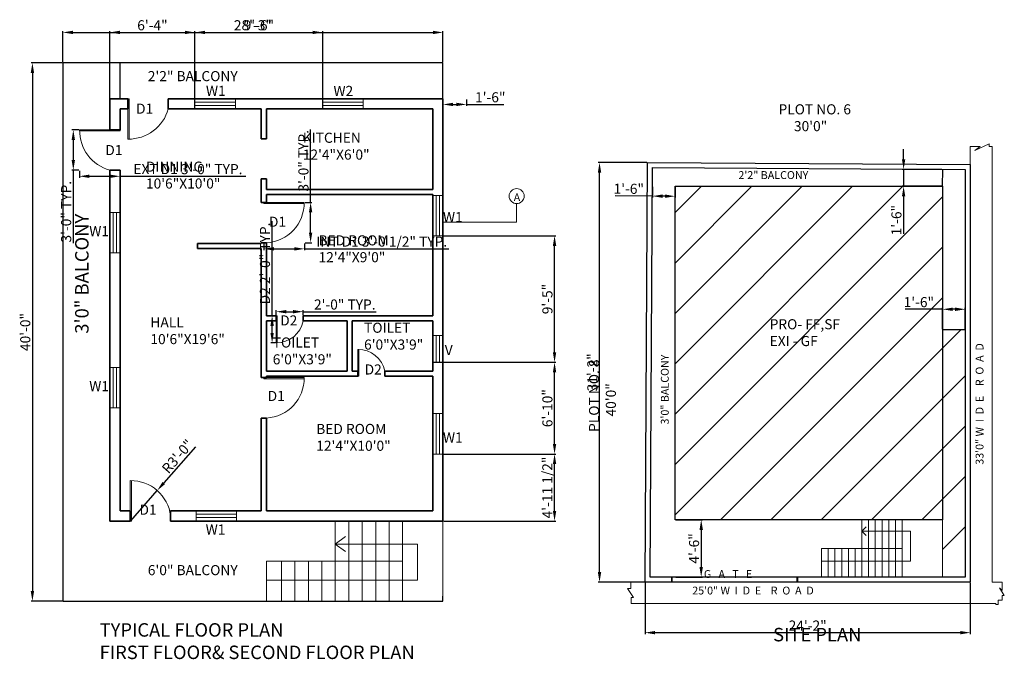
# Model space of a CAD drawing. Units: inches. Extents: x 2044 to 3644, y 808 to 1988.
# Tile 3 of 4: x 2766 to 3644, y 841 to 1412. Entities that reach past the tile are written whole.
import ezdxf

# ---------------------------------------------------------------- set-up
doc = ezdxf.new("R2010")
doc.units = ezdxf.units.IN
for name, color, linetype, lineweight in [('A-ANNO-DIMS', 2, 'Continuous', 18), ('A-ANNO-SYMB', 2, 'Continuous', 18), ('A-ANNO-TEXT', 7, 'Continuous', 18), ('A-ANNO-TITL', 7, 'Continuous', 25), ('A-AREA-IDEN', 7, 'Continuous', 18), ('A-DOOR', 4, 'Continuous', 18), ('A-FLOR-BALC', 7, 'Continuous', 25), ('A-FLOR-STRS', 3, 'Continuous', 18), ('A-GLAZ', 4, 'Continuous', 18), ('A-WALL', 7, 'Continuous', 35), ('C-BLDG', 7, 'Continuous', 25), ('C-BLDG-PATT', 252, 'Continuous', 13), ('C-PROP', 3, 'Continuous', 25), ('C-ROAD', 8, 'Continuous', 18)]:
    doc.layers.add(name, color=color, linetype=linetype, lineweight=lineweight)
doc.styles.get("Standard").update_dxf_attribs({"font": 'arial.ttf'})
doc.dimstyles.new('ISO-25', dxfattribs={"dimtxt": 9, "dimasz": 9, "dimexe": 1.25, "dimexo": 0.625, "dimtad": 1, "dimdec": 1, "dimrnd": 9, "dimlunit": 3, "dimtxsty": 'Standard', "dimcen": 2.5, "dimadec": 0, "dimazin": 0, "dimtfac": 1, "dimtdec": 1, "dimtmove": 0, "dimatfit": 3, "dimfxl": 1, "dimarcsym": 0})

# ---------------------------------------------------------------- blocks, each defined once
blk = doc.blocks.new('*D6')
at = {"layer": 'A-ANNO-DIMS', "color": 0, "lineweight": -2, "transparency": 16777216}
for p, q in [((3142.98, 1340.62), (3142.98, 1334.91)), ((3151.98, 1336.16), (3154.98, 1336.16)), ((3163.98, 1340.62), (3163.98, 1334.91)), ((3163.98, 1336.16), (3197.31, 1336.16))]:
    blk.add_line(p, q, dxfattribs=at)
at = {"layer": 'A-ANNO-DIMS', "color": 0, "transparency": 16777216}
for points in [[(3151.98, 1337.66), (3151.98, 1334.66), (3142.98, 1336.16)], [(3154.98, 1337.66), (3154.98, 1334.66), (3163.98, 1336.16)]]:
    blk.add_solid(points, dxfattribs=at)
at = {"layer": 'Defpoints', "color": 0, "transparency": 16777216}
for p in [(3142.98, 1341.25), (3163.98, 1341.25), (3163.98, 1336.16)]:
    blk.add_point(p, dxfattribs=at)
at = {"layer": 'A-ANNO-DIMS', "color": 0, "transparency": 16777216, "insert": (3185.14, 1341.38), "char_height": 9, "attachment_point": 5}
blk.add_mtext('1\'-6"', dxfattribs=at)
blk = doc.blocks.new('*D8')
at = {"layer": 'A-ANNO-DIMS', "color": 0, "lineweight": -2, "transparency": 16777216}
for p, q in [((3350.64, 965.86), (3374.52, 965.86)), ((3373.27, 956.86), (3373.27, 923.7)), ((3350.64, 914.7), (3374.52, 914.7))]:
    blk.add_line(p, q, dxfattribs=at)
at = {"layer": 'A-ANNO-DIMS', "color": 0, "transparency": 16777216}
for points in [[(3371.77, 956.86), (3374.77, 956.86), (3373.27, 965.86)], [(3371.77, 923.7), (3374.77, 923.7), (3373.27, 914.7)]]:
    blk.add_solid(points, dxfattribs=at)
at = {"layer": 'Defpoints', "color": 0, "transparency": 16777216}
for p in [(3350.02, 965.86), (3350.02, 914.7), (3373.27, 914.7)]:
    blk.add_point(p, dxfattribs=at)
at = {"layer": 'A-ANNO-DIMS', "color": 0, "transparency": 16777216, "insert": (3368.05, 940.28), "char_height": 9, "attachment_point": 5, "rotation": 90}
blk.add_mtext('4\'-6"', dxfattribs=at)
blk = doc.blocks.new('*D9')
at = {"layer": 'A-ANNO-DIMS', "color": 0, "lineweight": -2, "transparency": 16777216}
for p, q in [((3553.74, 1287.27), (3553.74, 1296.27)), ((3587.98, 1278.27), (3552.49, 1278.27)), ((3553.74, 1278.27), (3553.74, 1263.17)), ((3587.98, 1263.17), (3552.49, 1263.17)), ((3553.74, 1254.17), (3553.74, 1220.84))]:
    blk.add_line(p, q, dxfattribs=at)
at = {"layer": 'A-ANNO-DIMS', "color": 0, "transparency": 16777216}
for points in [[(3552.24, 1287.27), (3555.24, 1287.27), (3553.74, 1278.27)], [(3552.24, 1254.17), (3555.24, 1254.17), (3553.74, 1263.17)]]:
    blk.add_solid(points, dxfattribs=at)
at = {"layer": 'Defpoints', "color": 0, "transparency": 16777216}
for p in [(3588.61, 1278.27), (3553.74, 1263.17), (3588.61, 1263.17)]:
    blk.add_point(p, dxfattribs=at)
at = {"layer": 'A-ANNO-DIMS', "color": 0, "transparency": 16777216, "insert": (3548.52, 1233.01), "char_height": 9, "attachment_point": 5, "rotation": 90}
blk.add_mtext('1\'-6"', dxfattribs=at)
blk = doc.blocks.new('*D10')
at = {"layer": 'A-ANNO-DIMS', "color": 0, "lineweight": -2, "transparency": 16777216}
for p, q in [((3329.85, 1262.67), (3329.8, 1253.18)), ((3350.01, 1262.55), (3349.95, 1253.05)), ((3329.8, 1254.43), (3296.48, 1254.63)), ((3340.96, 1254.36), (3338.8, 1254.37))]:
    blk.add_line(p, q, dxfattribs=at)
at = {"layer": 'A-ANNO-DIMS', "color": 0, "transparency": 16777216}
for points in [[(3338.81, 1255.87), (3338.79, 1252.87), (3329.8, 1254.43)], [(3340.97, 1255.86), (3340.95, 1252.86), (3349.96, 1254.3)]]:
    blk.add_solid(points, dxfattribs=at)
at = {"layer": 'Defpoints', "color": 0, "transparency": 16777216}
for p in [(3329.86, 1263.3), (3350.02, 1263.17), (3329.8, 1254.43)]:
    blk.add_point(p, dxfattribs=at)
at = {"layer": 'A-ANNO-DIMS', "color": 0, "transparency": 16777216, "insert": (3308.67, 1259.78), "char_height": 9, "attachment_point": 5, "rotation": 359.64878}
blk.add_mtext('1\'-6"', dxfattribs=at)
blk = doc.blocks.new('*D11')
at = {"layer": 'A-ANNO-DIMS', "color": 0, "lineweight": -2, "transparency": 16777216}
for p, q in [((3588.52, 1153.52), (3555.19, 1153.52)), ((3588.52, 1135.78), (3588.52, 1154.77)), ((3599.7, 1153.52), (3597.52, 1153.52)), ((3608.7, 1135.78), (3608.7, 1154.77))]:
    blk.add_line(p, q, dxfattribs=at)
at = {"layer": 'A-ANNO-DIMS', "color": 0, "transparency": 16777216}
for points in [[(3597.52, 1155.02), (3597.52, 1152.02), (3588.52, 1153.52)], [(3599.7, 1155.02), (3599.7, 1152.02), (3608.7, 1153.52)]]:
    blk.add_solid(points, dxfattribs=at)
at = {"layer": 'Defpoints', "color": 0, "transparency": 16777216}
for p in [(3588.52, 1153.52), (3588.52, 1135.15), (3608.7, 1135.15)]:
    blk.add_point(p, dxfattribs=at)
at = {"layer": 'A-ANNO-DIMS', "color": 0, "transparency": 16777216, "insert": (3567.35, 1158.74), "char_height": 9, "attachment_point": 5}
blk.add_mtext('1\'-6"', dxfattribs=at)
blk = doc.blocks.new('DOOR-D1-36-EXT')
for p, q in [((0, 36), (1, 36)), ((1, 36), (1, 0)), ((0, 0), (0, 27)), ((1, 0), (0, 0))]:
    blk.add_line(p, q)
blk.add_arc((0.5, 36.83), 36.84, 269.22228, 344.51752)
blk = doc.blocks.new('DOOR-D1-36-INT')
for p, q in [((0, 36), (0, 35)), ((36, 36), (2.25, 36)), ((36, 35), (36, 36)), ((0, 35), (36, 35))]:
    blk.add_line(p, q)
blk.add_arc((0.46, 35.5), 35.55, 272.88924, 0.80598)
blk = doc.blocks.new('DOOR-D2-24')
for p, q in [((0, 24), (1, 24)), ((0, 0), (0, 19.5)), ((1, 24), (1, 0)), ((1, 0), (0, 0))]:
    blk.add_line(p, q)
blk.add_arc((0.5, 23.9), 23.91, 268.80171, 349.38601)
blk = doc.blocks.new('WIN-W1-36')
for p, q in [((0, 9), (0, 0)), ((36, 9), (36, 0)), ((36, 6), (0, 6)), ((36, 3), (0, 3))]:
    blk.add_line(p, q)
blk = doc.blocks.new('WIN-W2-36')
for p, q in [((0, 9), (0, 0)), ((36, 9), (36, 0)), ((36, 6), (0, 6)), ((36, 3), (0, 3))]:
    blk.add_line(p, q)
blk = doc.blocks.new('VENT-24')
for p, q in [((0, 24), (9, 24)), ((3, 0), (3, 24)), ((6, 0), (6, 24)), ((0, 0), (9, 0))]:
    blk.add_line(p, q)
blk = doc.blocks.new('STAIR-RETURN-PLAN')
for p, q in [((61.5, 71.5), (61.5, 0)), ((73.5, 71.5), (73.5, 0)), ((85.5, 71.5), (85.5, 0)), ((97.5, 71.5), (97.5, 0)), ((109.5, 71.5), (109.5, 0)), ((121.5, 71.5), (121.5, 0)), ((61.5, 50.86), (70.45, 57.63)), ((134.75, 50.86), (61.5, 50.86)), ((61.5, 50.86), (70.45, 44.26)), ((134.75, 18.82), (134.75, 50.86)), ((0, 35.75), (0, 0)), ((121.5, 35.75), (0, 35.75)), ((13.5, 35.75), (13.5, 0)), ((25.5, 35.75), (25.5, 0)), ((37.5, 35.75), (37.5, 0)), ((49.5, 35.75), (49.5, 0)), ((0, 18.82), (134.75, 18.82))]:
    blk.add_line(p, q)
blk = doc.blocks.new('SECTION-MARK-ELBOW')
for p, q in [((6.87, 0), (6.87, 16.52)), ((72.41, 0), (6.87, 0))]:
    blk.add_line(p, q)
blk.add_circle((6.7, 23.26), 6.7)
blk = doc.blocks.new('*D33')
at = {"layer": 'A-ANNO-DIMS', "color": 0, "lineweight": -2, "transparency": 16777216}
for p, q in [((2818.75, 1276.9), (2818.75, 1270.84)), ((2854.98, 1276.9), (2854.98, 1270.84)), ((2827.75, 1272.09), (2845.98, 1272.09)), ((2854.98, 1272.09), (2967.13, 1272.09))]:
    blk.add_line(p, q, dxfattribs=at)
at = {"layer": 'A-ANNO-DIMS', "color": 0, "transparency": 16777216}
for points in [[(2827.75, 1273.59), (2827.75, 1270.59), (2818.75, 1272.09)], [(2845.98, 1273.59), (2845.98, 1270.59), (2854.98, 1272.09)]]:
    blk.add_solid(points, dxfattribs=at)
at = {"layer": 'Defpoints', "color": 0, "transparency": 16777216}
for p in [(2818.75, 1277.53), (2854.98, 1277.53), (2854.98, 1272.09)]:
    blk.add_point(p, dxfattribs=at)
at = {"layer": 'A-ANNO-DIMS', "color": 0, "transparency": 16777216, "insert": (2915.56, 1277.32), "char_height": 9, "attachment_point": 5}
blk.add_mtext('EXT D1 3\'-0" TYP.', dxfattribs=at)
blk = doc.blocks.new('*D34')
at = {"layer": 'A-ANNO-DIMS', "color": 0, "lineweight": -2, "transparency": 16777216}
for p, q in [((2818.13, 1313.53), (2812.07, 1313.53)), ((2813.32, 1304.53), (2813.32, 1286.53)), ((2818.13, 1277.53), (2812.07, 1277.53)), ((2813.32, 1277.53), (2813.32, 1212.42))]:
    blk.add_line(p, q, dxfattribs=at)
at = {"layer": 'A-ANNO-DIMS', "color": 0, "transparency": 16777216}
for points in [[(2811.82, 1304.53), (2814.82, 1304.53), (2813.32, 1313.53)], [(2811.82, 1286.53), (2814.82, 1286.53), (2813.32, 1277.53)]]:
    blk.add_solid(points, dxfattribs=at)
at = {"layer": 'Defpoints', "color": 0, "transparency": 16777216}
for p in [(2818.75, 1313.53), (2813.32, 1277.53), (2818.75, 1277.53)]:
    blk.add_point(p, dxfattribs=at)
at = {"layer": 'A-ANNO-DIMS', "color": 0, "transparency": 16777216, "insert": (2808.1, 1240.48), "char_height": 9, "attachment_point": 5, "rotation": 90}
blk.add_mtext('3\'-0" TYP.', dxfattribs=at)
blk = doc.blocks.new('*D35')
at = {"layer": 'A-ANNO-DIMS', "color": 0, "lineweight": -2, "transparency": 16777216}
for p, q in [((2983.23, 1212.22), (2983.23, 1206.16)), ((3019.5, 1212.22), (3019.5, 1206.16)), ((2992.23, 1207.41), (3010.5, 1207.41)), ((3019.5, 1207.41), (3148.24, 1207.41))]:
    blk.add_line(p, q, dxfattribs=at)
at = {"layer": 'A-ANNO-DIMS', "color": 0, "transparency": 16777216}
for points in [[(2992.23, 1208.91), (2992.23, 1205.91), (2983.23, 1207.41)], [(3010.5, 1208.91), (3010.5, 1205.91), (3019.5, 1207.41)]]:
    blk.add_solid(points, dxfattribs=at)
at = {"layer": 'Defpoints', "color": 0, "transparency": 16777216}
for p in [(2983.23, 1212.85), (3019.5, 1212.85), (3019.5, 1207.41)]:
    blk.add_point(p, dxfattribs=at)
at = {"layer": 'A-ANNO-DIMS', "color": 0, "transparency": 16777216, "insert": (3088.37, 1212.69), "char_height": 9, "attachment_point": 5}
blk.add_mtext('INT D1 3\'-0 1/2" TYP.', dxfattribs=at)
blk = doc.blocks.new('*D36')
at = {"layer": 'A-ANNO-DIMS', "color": 0, "lineweight": -2, "transparency": 16777216}
for p, q in [((3024.94, 1248.85), (3024.94, 1313.95)), ((3020.13, 1248.85), (3026.19, 1248.85)), ((3024.94, 1221.85), (3024.94, 1239.85)), ((3020.13, 1212.85), (3026.19, 1212.85))]:
    blk.add_line(p, q, dxfattribs=at)
at = {"layer": 'A-ANNO-DIMS', "color": 0, "transparency": 16777216}
for points in [[(3023.44, 1239.85), (3026.44, 1239.85), (3024.94, 1248.85)], [(3023.44, 1221.85), (3026.44, 1221.85), (3024.94, 1212.85)]]:
    blk.add_solid(points, dxfattribs=at)
at = {"layer": 'Defpoints', "color": 0, "transparency": 16777216}
for p in [(3019.5, 1248.85), (3024.94, 1248.85), (3019.5, 1212.85)]:
    blk.add_point(p, dxfattribs=at)
at = {"layer": 'A-ANNO-DIMS', "color": 0, "transparency": 16777216, "insert": (3019.72, 1285.9), "char_height": 9, "attachment_point": 5, "rotation": 90}
blk.add_mtext('3\'-0" TYP.', dxfattribs=at)
blk = doc.blocks.new('*D37')
at = {"layer": 'A-ANNO-DIMS', "color": 0, "lineweight": -2, "transparency": 16777216}
for p, q in [((2990.63, 1147.75), (2990.63, 1231.97)), ((2993.65, 1147.75), (2989.38, 1147.75)), ((2990.63, 1132.5), (2990.63, 1138.75)), ((2993.65, 1123.5), (2989.38, 1123.5))]:
    blk.add_line(p, q, dxfattribs=at)
at = {"layer": 'A-ANNO-DIMS', "color": 0, "transparency": 16777216}
for points in [[(2989.13, 1138.75), (2992.13, 1138.75), (2990.63, 1147.75)], [(2989.13, 1132.5), (2992.13, 1132.5), (2990.63, 1123.5)]]:
    blk.add_solid(points, dxfattribs=at)
at = {"layer": 'Defpoints', "color": 0, "transparency": 16777216}
for p in [(2990.63, 1147.75), (2994.27, 1147.75), (2994.27, 1123.5)]:
    blk.add_point(p, dxfattribs=at)
at = {"layer": 'A-ANNO-DIMS', "color": 0, "transparency": 16777216, "insert": (2985.41, 1194.36), "char_height": 9, "attachment_point": 5, "rotation": 90}
blk.add_mtext('D2 2\'-0" TYP.', dxfattribs=at)
blk = doc.blocks.new('*D38')
at = {"layer": 'A-ANNO-DIMS', "color": 0, "lineweight": -2, "transparency": 16777216}
for p, q in [((2994.27, 1148.37), (2994.27, 1152.63)), ((3003.27, 1151.38), (3009.27, 1151.38)), ((3018.27, 1148.37), (3018.27, 1152.63)), ((3018.27, 1151.38), (3083.53, 1151.38))]:
    blk.add_line(p, q, dxfattribs=at)
at = {"layer": 'A-ANNO-DIMS', "color": 0, "transparency": 16777216}
for points in [[(3003.27, 1152.88), (3003.27, 1149.88), (2994.27, 1151.38)], [(3009.27, 1152.88), (3009.27, 1149.88), (3018.27, 1151.38)]]:
    blk.add_solid(points, dxfattribs=at)
at = {"layer": 'Defpoints', "color": 0, "transparency": 16777216}
for p in [(3018.27, 1151.38), (2994.27, 1147.75), (3018.27, 1147.75)]:
    blk.add_point(p, dxfattribs=at)
at = {"layer": 'A-ANNO-DIMS', "color": 0, "transparency": 16777216, "insert": (3055.4, 1156.6), "char_height": 9, "attachment_point": 5}
blk.add_mtext('2\'-0" TYP.', dxfattribs=at)
blk = doc.blocks.new('*D53')
at = {"layer": 'A-ANNO-DIMS', "color": 0, "lineweight": -2, "transparency": 16777216}
for p, q in [((2803.98, 1373.87), (2803.98, 1401.6)), ((2812.98, 1400.35), (3133.98, 1400.35)), ((3142.98, 1373.87), (3142.98, 1401.6))]:
    blk.add_line(p, q, dxfattribs=at)
at = {"layer": 'A-ANNO-DIMS', "color": 0, "transparency": 16777216}
for points in [[(2812.98, 1401.85), (2812.98, 1398.85), (2803.98, 1400.35)], [(3133.98, 1401.85), (3133.98, 1398.85), (3142.98, 1400.35)]]:
    blk.add_solid(points, dxfattribs=at)
at = {"layer": 'Defpoints', "color": 0, "transparency": 16777216}
for p in [(3142.98, 1400.35), (2803.98, 1373.25), (3142.98, 1373.25)]:
    blk.add_point(p, dxfattribs=at)
at = {"layer": 'A-ANNO-DIMS', "color": 0, "transparency": 16777216, "insert": (2973.48, 1405.57), "char_height": 9, "attachment_point": 5}
blk.add_mtext('28\'-3"', dxfattribs=at)
blk = doc.blocks.new('*D54')
at = {"layer": 'A-ANNO-DIMS', "color": 0, "lineweight": -2, "transparency": 16777216}
for p, q in [((2803.36, 1373.25), (2775.63, 1373.25)), ((2776.88, 1364.25), (2776.88, 902.25)), ((2803.36, 893.25), (2775.63, 893.25))]:
    blk.add_line(p, q, dxfattribs=at)
at = {"layer": 'A-ANNO-DIMS', "color": 0, "transparency": 16777216}
for points in [[(2775.38, 1364.25), (2778.38, 1364.25), (2776.88, 1373.25)], [(2775.38, 902.25), (2778.38, 902.25), (2776.88, 893.25)]]:
    blk.add_solid(points, dxfattribs=at)
at = {"layer": 'Defpoints', "color": 0, "transparency": 16777216}
for p in [(2803.98, 1373.25), (2776.88, 893.25), (2803.98, 893.25)]:
    blk.add_point(p, dxfattribs=at)
at = {"layer": 'A-ANNO-DIMS', "color": 0, "transparency": 16777216, "insert": (2771.66, 1133.25), "char_height": 9, "attachment_point": 5, "rotation": 90}
blk.add_mtext('40\'-0"', dxfattribs=at)
blk = doc.blocks.new('*D55')
at = {"layer": 'A-ANNO-DIMS', "color": 0, "lineweight": -2, "transparency": 16777216}
for p, q in [((2845.98, 1341.87), (2845.98, 1401.6)), ((2854.98, 1400.35), (2912.83, 1400.35)), ((2921.83, 1332.87), (2921.83, 1401.6))]:
    blk.add_line(p, q, dxfattribs=at)
at = {"layer": 'A-ANNO-DIMS', "color": 0, "transparency": 16777216}
for points in [[(2854.98, 1401.85), (2854.98, 1398.85), (2845.98, 1400.35)], [(2912.83, 1401.85), (2912.83, 1398.85), (2921.83, 1400.35)]]:
    blk.add_solid(points, dxfattribs=at)
at = {"layer": 'Defpoints', "color": 0, "transparency": 16777216}
for p in [(2921.83, 1400.35), (2845.98, 1341.25), (2921.83, 1332.25)]:
    blk.add_point(p, dxfattribs=at)
at = {"layer": 'A-ANNO-DIMS', "color": 0, "transparency": 16777216, "insert": (2883.9, 1405.57), "char_height": 9, "attachment_point": 5}
blk.add_mtext('6\'-4"', dxfattribs=at)
blk = doc.blocks.new('*D56')
at = {"layer": 'A-ANNO-DIMS', "color": 0, "lineweight": -2, "transparency": 16777216}
for p, q in [((2921.83, 1332.87), (2921.83, 1401.6)), ((2930.83, 1400.35), (3026.77, 1400.35)), ((3035.77, 1332.87), (3035.77, 1401.6))]:
    blk.add_line(p, q, dxfattribs=at)
at = {"layer": 'A-ANNO-DIMS', "color": 0, "transparency": 16777216}
for points in [[(2930.83, 1401.85), (2930.83, 1398.85), (2921.83, 1400.35)], [(3026.77, 1401.85), (3026.77, 1398.85), (3035.77, 1400.35)]]:
    blk.add_solid(points, dxfattribs=at)
at = {"layer": 'Defpoints', "color": 0, "transparency": 16777216}
for p in [(3035.77, 1400.35), (2921.83, 1332.25), (3035.77, 1332.25)]:
    blk.add_point(p, dxfattribs=at)
at = {"layer": 'A-ANNO-DIMS', "color": 0, "transparency": 16777216, "insert": (2978.8, 1405.57), "char_height": 9, "attachment_point": 5}
blk.add_mtext('9\'-6"', dxfattribs=at)
blk = doc.blocks.new('*D57')
at = {"layer": 'A-ANNO-DIMS', "color": 0, "lineweight": -2, "transparency": 16777216}
for p, q in [((3143.61, 1024.48), (3243.74, 1024.48)), ((3242.49, 973.75), (3242.49, 1015.48)), ((3143.61, 964.75), (3243.74, 964.75))]:
    blk.add_line(p, q, dxfattribs=at)
at = {"layer": 'A-ANNO-DIMS', "color": 0, "transparency": 16777216}
for points in [[(3240.99, 1015.48), (3243.99, 1015.48), (3242.49, 1024.48)], [(3240.99, 973.75), (3243.99, 973.75), (3242.49, 964.75)]]:
    blk.add_solid(points, dxfattribs=at)
at = {"layer": 'Defpoints', "color": 0, "transparency": 16777216}
for p in [(3142.98, 1024.48), (3242.49, 1024.48), (3142.98, 964.75)]:
    blk.add_point(p, dxfattribs=at)
at = {"layer": 'A-ANNO-DIMS', "color": 0, "transparency": 16777216, "insert": (3237.21, 994.61), "char_height": 9, "attachment_point": 5, "rotation": 90}
blk.add_mtext('4\'-11 1/2"', dxfattribs=at)
blk = doc.blocks.new('*D58')
at = {"layer": 'A-ANNO-DIMS', "color": 0, "lineweight": -2, "transparency": 16777216}
for p, q in [((3134.61, 1106.26), (3243.74, 1106.26)), ((3242.49, 1033.48), (3242.49, 1097.26)), ((3143.61, 1024.48), (3243.74, 1024.48))]:
    blk.add_line(p, q, dxfattribs=at)
at = {"layer": 'A-ANNO-DIMS', "color": 0, "transparency": 16777216}
for points in [[(3240.99, 1097.26), (3243.99, 1097.26), (3242.49, 1106.26)], [(3240.99, 1033.48), (3243.99, 1033.48), (3242.49, 1024.48)]]:
    blk.add_solid(points, dxfattribs=at)
at = {"layer": 'Defpoints', "color": 0, "transparency": 16777216}
for p in [(3133.98, 1106.26), (3242.49, 1106.26), (3142.98, 1024.48)]:
    blk.add_point(p, dxfattribs=at)
at = {"layer": 'A-ANNO-DIMS', "color": 0, "transparency": 16777216, "insert": (3237.27, 1065.37), "char_height": 9, "attachment_point": 5, "rotation": 90}
blk.add_mtext('6\'-10"', dxfattribs=at)
blk = doc.blocks.new('*D59')
at = {"layer": 'A-ANNO-DIMS', "color": 0, "lineweight": -2, "transparency": 16777216}
for p, q in [((3143.61, 1219.03), (3243.74, 1219.03)), ((3242.49, 1115.26), (3242.49, 1210.03)), ((3134.61, 1106.26), (3243.74, 1106.26))]:
    blk.add_line(p, q, dxfattribs=at)
at = {"layer": 'A-ANNO-DIMS', "color": 0, "transparency": 16777216}
for points in [[(3240.99, 1210.03), (3243.99, 1210.03), (3242.49, 1219.03)], [(3240.99, 1115.26), (3243.99, 1115.26), (3242.49, 1106.26)]]:
    blk.add_solid(points, dxfattribs=at)
at = {"layer": 'Defpoints', "color": 0, "transparency": 16777216}
for p in [(3142.98, 1219.03), (3242.49, 1219.03), (3133.98, 1106.26)]:
    blk.add_point(p, dxfattribs=at)
at = {"layer": 'A-ANNO-DIMS', "color": 0, "transparency": 16777216, "insert": (3237.27, 1162.65), "char_height": 9, "attachment_point": 5, "rotation": 90}
blk.add_mtext('9\'-5"', dxfattribs=at)
blk = doc.blocks.new('*D60')
at = {"layer": 'A-ANNO-DIMS', "color": 0, "lineweight": -2, "transparency": 16777216}
for p, q in [((3323.19, 909.57), (3323.19, 863.96)), ((3613.2, 909.57), (3613.2, 863.96)), ((3332.19, 865.21), (3604.2, 865.21))]:
    blk.add_line(p, q, dxfattribs=at)
at = {"layer": 'A-ANNO-DIMS', "color": 0, "transparency": 16777216}
for points in [[(3332.19, 866.71), (3332.19, 863.71), (3323.19, 865.21)], [(3604.2, 866.71), (3604.2, 863.71), (3613.2, 865.21)]]:
    blk.add_solid(points, dxfattribs=at)
at = {"layer": 'Defpoints', "color": 0, "transparency": 16777216}
for p in [(3323.19, 910.2), (3613.2, 910.2), (3613.2, 865.21)]:
    blk.add_point(p, dxfattribs=at)
at = {"layer": 'A-ANNO-DIMS', "color": 0, "transparency": 16777216, "insert": (3468.2, 870.35), "char_height": 9, "attachment_point": 5}
blk.add_mtext('24\'-2"', dxfattribs=at)
blk = doc.blocks.new('*D61')
at = {"layer": 'A-ANNO-DIMS', "color": 0, "lineweight": -2, "transparency": 16777216}
for p, q in [((3324.86, 1284.38), (3281.33, 1284.38)), ((3282.58, 919.2), (3282.58, 1275.38)), ((3322.57, 910.2), (3281.33, 910.2))]:
    blk.add_line(p, q, dxfattribs=at)
at = {"layer": 'A-ANNO-DIMS', "color": 0, "transparency": 16777216}
for points in [[(3281.08, 1275.38), (3284.08, 1275.38), (3282.58, 1284.38)], [(3281.08, 919.2), (3284.08, 919.2), (3282.58, 910.2)]]:
    blk.add_solid(points, dxfattribs=at)
at = {"layer": 'Defpoints', "color": 0, "transparency": 16777216}
for p in [(3282.58, 1284.38), (3325.49, 1284.38), (3323.19, 910.2)]:
    blk.add_point(p, dxfattribs=at)
at = {"layer": 'A-ANNO-DIMS', "color": 0, "transparency": 16777216, "insert": (3277.36, 1097.29), "char_height": 9, "attachment_point": 5, "rotation": 90}
blk.add_mtext('31\'-2"', dxfattribs=at)
blk = doc.blocks.new('*D77')
at = {"layer": 'A-ANNO-DIMS', "color": 0, "lineweight": -2, "transparency": 16777216}
for p, q in [((2922.25, 1030.88), (2894.07, 998.68)), ((2864.6, 965), (2888.15, 991.91))]:
    blk.add_line(p, q, dxfattribs=at)
at = {"layer": 'A-ANNO-DIMS', "color": 0, "transparency": 16777216}
blk.add_solid([(2892.95, 999.67), (2895.2, 997.69), (2888.15, 991.91)], dxfattribs=at)
at = {"layer": 'Defpoints', "color": 0, "transparency": 16777216}
for p in [(2888.15, 991.91), (2864.6, 965)]:
    blk.add_point(p, dxfattribs=at)
at = {"layer": 'A-ANNO-DIMS', "color": 0, "transparency": 16777216, "insert": (2907.19, 1021.61), "char_height": 9, "attachment_point": 5, "rotation": 48.81443}
blk.add_mtext('R3\'-0"', dxfattribs=at)

msp = doc.modelspace()

# ---------------------------------------------------------------- hatches: boundary and pattern name
at = {"layer": 'C-BLDG-PATT'}
h = msp.add_hatch(dxfattribs=at)
h.set_pattern_fill('ANSI31', color=256, scale=10)
h.paths.add_polyline_path([(3588.52, 1263.17), (3350.02, 1263.17), (3350.02, 965.86), (3588.52, 965.86)])
h.paths.add_polyline_path([(3608.7, 1135.15), (3588.52, 1135.15), (3588.52, 965.86), (3588.52, 914.7), (3608.7, 914.7)])
h.paths.add_polyline_path([(3557.87, 1222.04), (3557.87, 1247.39), (3539.33, 1247.39), (3539.33, 1222.04)], flags=24)
h.paths.add_polyline_path([(3431.07, 1115.47), (3505.44, 1115.47), (3505.44, 1149.17), (3431.07, 1149.17)], flags=24)

# ---------------------------------------------------------------- linework, layer by layer
at = {"layer": 'A-DOOR'}
for p, q in [((2864.1, 1000.75), (2864.1, 973.75)), ((2865.1, 964.75), (2865.1, 1000.75)), ((2864.1, 964.75), (2865.1, 964.75))]:
    msp.add_line(p, q, dxfattribs=at)
msp.add_arc((2864.6, 965), 35.75, 6.82686, 90.80129, dxfattribs=at)
at = {"layer": 'A-FLOR-BALC'}
for p, q in [((3142.98, 1373.25), (2803.98, 1373.25)), ((2803.98, 1373.25), (2803.98, 893.25)), ((2845.98, 1341.25), (2845.98, 1373.25)), ((2854.98, 1341.25), (2854.98, 1373.25)), ((3142.98, 1341.25), (3142.98, 1373.25)), ((3142.98, 893.25), (3142.98, 897.75)), ((2803.98, 893.25), (3142.98, 893.25))]:
    msp.add_line(p, q, dxfattribs=at)
at = {"layer": 'A-FLOR-STRS'}
for p, q in [((3516.52, 965.86), (3516.52, 914.7)), ((3522.52, 965.86), (3522.52, 914.7)), ((3528.52, 965.86), (3528.52, 914.7)), ((3534.52, 965.86), (3534.52, 914.7)), ((3540.52, 965.86), (3540.52, 914.7)), ((3546.52, 965.86), (3546.52, 914.7)), ((3546.52, 965.86), (3546.52, 914.7)), ((3552.52, 965.86), (3552.52, 914.7)), ((3588.52, 965.86), (3588.52, 914.7)), ((3142.98, 964.75), (3142.98, 893.25)), ((3516.52, 955.67), (3520.38, 959.45)), ((3560, 955.67), (3516.52, 955.67)), ((3516.52, 955.67), (3520.38, 951.73)), ((3560, 928.92), (3560, 955.67)), ((3480.52, 940.28), (3480.52, 914.7)), ((3552.52, 940.28), (3480.52, 940.28)), ((3486.52, 940.28), (3486.52, 914.7)), ((3492.52, 940.28), (3492.52, 914.7)), ((3498.52, 940.28), (3498.52, 914.7)), ((3504.52, 940.28), (3504.52, 914.7)), ((3510.52, 940.28), (3510.52, 914.7)), ((3480.52, 928.92), (3560, 928.92))]:
    msp.add_line(p, q, dxfattribs=at)
at = {"layer": 'A-WALL'}
for p, q in [((2862.06, 1341.25), (2845.98, 1341.25)), ((2845.98, 1341.25), (2845.98, 1313.53)), ((2862.06, 1341.25), (2862.06, 1332.25)), ((3142.98, 1341.25), (2898.06, 1341.25)), ((2898.06, 1341.25), (2898.06, 1332.25)), ((3142.98, 964.75), (3142.98, 1341.25)), ((2862.06, 1332.25), (2854.98, 1332.25)), ((2854.98, 1332.25), (2854.98, 1313.53)), ((2980.98, 1332.25), (2898.06, 1332.25)), ((2980.98, 1332.25), (2980.98, 1305.52)), ((3133.98, 1332.25), (2985.48, 1332.25)), ((2985.48, 1332.25), (2985.48, 1305.52)), ((3133.98, 1260.25), (3133.98, 1332.25)), ((2854.98, 1313.53), (2845.98, 1313.53)), ((2985.48, 1305.52), (2980.98, 1305.52)), ((2845.98, 1277.53), (2845.98, 1042.75)), ((2854.98, 1277.53), (2845.98, 1277.53)), ((2854.98, 1277.53), (2854.98, 1212.25)), ((2980.98, 1269.95), (2980.98, 1248.85)), ((2985.48, 1269.95), (2980.98, 1269.95)), ((2985.48, 1269.95), (2985.48, 1260.25)), ((3133.98, 1260.25), (2985.48, 1260.25)), ((3133.98, 1255.75), (2985.48, 1255.75)), ((2985.48, 1255.75), (2985.48, 1248.85)), ((3133.98, 1147.75), (3133.98, 1255.75)), ((2985.48, 1248.85), (2980.98, 1248.85)), ((2854.98, 1212.25), (2854.98, 1207.75)), ((2980.98, 1212.25), (2924.1, 1212.25)), ((2924.1, 1212.25), (2924.1, 1207.75)), ((2980.98, 1212.85), (2980.98, 1212.25)), ((2985.48, 1212.85), (2980.98, 1212.85)), ((2985.48, 1212.85), (2985.48, 1147.75)), ((2854.98, 1207.75), (2854.98, 1051.75)), ((2980.98, 1207.75), (2924.1, 1207.75)), ((2980.98, 1207.75), (2980.98, 1092.57)), ((2994.27, 1147.75), (2985.48, 1147.75)), ((2994.27, 1143.25), (2985.48, 1143.25)), ((2985.48, 1143.25), (2985.48, 1098.25)), ((2994.27, 1147.75), (2994.27, 1143.25)), ((3133.98, 1147.75), (3018.27, 1147.75)), ((3018.27, 1147.75), (3018.27, 1143.25)), ((3057.48, 1143.25), (3018.27, 1143.25)), ((3057.48, 1098.25), (3057.48, 1143.25)), ((3061.98, 1098.25), (3061.98, 1143.25)), ((3133.98, 1143.25), (3061.98, 1143.25)), ((3133.98, 1098.25), (3133.98, 1143.25)), ((3057.48, 1098.25), (2985.48, 1098.25)), ((3067.08, 1098.25), (3061.98, 1098.25)), ((3067.08, 1098.25), (3067.08, 1093.75)), ((3133.98, 1098.25), (3091.08, 1098.25)), ((3091.08, 1098.25), (3091.08, 1093.75)), ((2985.48, 1092.57), (2980.98, 1092.57)), ((3067.08, 1093.75), (2985.48, 1093.75)), ((2985.48, 1093.75), (2985.48, 1092.57)), ((3133.98, 1093.75), (3091.08, 1093.75)), ((3133.98, 973.75), (3133.98, 1093.75)), ((2980.98, 1056.57), (2980.98, 1051.75)), ((2985.48, 1056.57), (2980.98, 1056.57)), ((2985.48, 1056.57), (2985.48, 973.75)), ((2854.98, 1051.75), (2854.98, 973.75)), ((2980.98, 1051.75), (2980.98, 1042.75)), ((2845.98, 1042.75), (2845.98, 964.75)), ((2980.98, 1042.75), (2980.98, 973.75)), ((2864.1, 973.75), (2854.98, 973.75)), ((2864.1, 973.75), (2864.1, 964.75)), ((2980.98, 973.75), (2900.1, 973.75)), ((2900.1, 973.75), (2900.1, 964.75)), ((3133.98, 973.75), (2985.48, 973.75)), ((2864.1, 964.75), (2845.98, 964.75)), ((2980.98, 964.75), (2900.1, 964.75)), ((3142.98, 964.75), (2980.98, 964.75))]:
    msp.add_line(p, q, dxfattribs=at)
at = {"layer": 'C-BLDG'}
for p, q in [((3588.52, 1263.17), (3588.61, 1278.27)), ((3608.7, 1135.15), (3588.52, 1135.15))]:
    msp.add_line(p, q, dxfattribs=at)
msp.add_lwpolyline([(3350.02, 1263.17), (3588.52, 1263.17), (3588.52, 965.86), (3350.02, 965.86)], close=True, dxfattribs=at)
at = {"layer": 'C-PROP'}
for p, q in [((3323.19, 910.2), (3325.49, 1284.38)), ((3325.49, 1284.38), (3613.2, 1282.61)), ((3613.2, 1282.61), (3613.2, 910.2)), ((3327.72, 914.7), (3329.96, 1279.85)), ((3329.96, 1279.85), (3608.7, 1278.14)), ((3608.7, 1278.14), (3608.7, 914.7)), ((3323.22, 914.7), (3323.19, 914.7)), ((3608.7, 914.7), (3327.72, 914.7)), ((3346.68, 914.7), (3346.68, 910.2)), ((3347.16, 914.7), (3347.16, 910.2)), ((3458.68, 914.7), (3458.68, 910.2)), ((3459.2, 914.7), (3459.2, 910.2)), ((3613.2, 910.2), (3323.19, 910.2)), ((3327.69, 910.17), (3327.69, 910.2))]:
    msp.add_line(p, q, dxfattribs=at)
at = {"layer": 'C-ROAD'}
for p, q in [((3617.39, 1295.11), (3629.96, 1300.97)), ((3629.96, 1300.97), (3629.96, 1298.55)), ((3613.2, 1282.61), (3613.2, 1298.55)), ((3613.2, 1298.55), (3621.98, 1298.55)), ((3621.98, 1298.55), (3617.39, 1295.11)), ((3629.96, 1298.55), (3632.64, 1298.55)), ((3632.64, 1298.55), (3632.64, 910.2)), ((3312.9, 896.53), (3307.68, 904.43)), ((3307.68, 904.43), (3310.64, 904.43)), ((3310.64, 904.43), (3310.64, 910.28)), ((3310.64, 910.28), (3323.19, 910.2)), ((3632.64, 910.2), (3641.57, 910.2)), ((3641.57, 902.75), (3639.37, 905.28)), ((3639.37, 905.28), (3643.55, 898.24)), ((3641.57, 910.2), (3641.57, 902.75)), ((3310.93, 891.18), (3310.93, 896.53)), ((3310.93, 896.53), (3312.9, 896.53)), ((3643.55, 898.24), (3641.57, 898.24)), ((3641.57, 898.24), (3641.57, 894.21)), ((3636.06, 891.18), (3310.93, 891.18)), ((3636.06, 890.31), (3636.06, 891.18)), ((3638.15, 890.31), (3636.06, 890.31)), ((3641.57, 894.21), (3638.15, 894.21)), ((3638.15, 894.21), (3638.15, 890.31))]:
    msp.add_line(p, q, dxfattribs=at)

# ---------------------------------------------------------------- block references
at = {"layer": 'A-ANNO-SYMB', "extrusion": (0, 0, -1), "zscale": -1}
msp.add_blockref('SECTION-MARK-ELBOW', (-3215.39, 1231.18), dxfattribs=at)
at = {"layer": 'A-DOOR'}
for name, p in [('DOOR-D1-36-EXT', (2862.06, 1305.25)), ('DOOR-D1-36-INT', (2983.23, 1212.85)), ('DOOR-D2-24', (2994.27, 1123.75)), ('DOOR-D1-36-INT', (2983.23, 1056.57))]:
    msp.add_blockref(name, p, dxfattribs=at)
at = {"layer": 'A-DOOR', "rotation": 269.9999999999993}
msp.add_blockref('DOOR-D1-36-EXT', (2818.98, 1313.53), dxfattribs=at)
at = {"layer": 'A-DOOR', "extrusion": (0, 0, -1), "zscale": -1, "rotation": 180}
msp.add_blockref('DOOR-D2-24', (-3067.08, 1117.75), dxfattribs=at)
at = {"layer": 'A-FLOR-STRS'}
msp.add_blockref('STAIR-RETURN-PLAN', (2985.48, 893.25), dxfattribs=at)
at = {"layer": 'A-GLAZ'}
for name, p in [('WIN-W1-36', (2921.83, 1332.25)), ('WIN-W2-36', (3035.77, 1332.25)), ('VENT-24', (3133.98, 1106.26)), ('WIN-W1-36', (2922.95, 964.75))]:
    msp.add_blockref(name, p, dxfattribs=at)
for p, rotation in [((3142.98, 1219.03), 90.00000000000003), ((2854.98, 1203.86), 89.99999999999984), ((2854.98, 1065.69), 90.00000000000138), ((3142.98, 1024.48), 90.00000000000053)]:
    msp.add_blockref('WIN-W1-36', p, dxfattribs=dict(at, rotation=rotation))

# ---------------------------------------------------------------- texts
at = {"layer": 'A-ANNO-SYMB', "insert": (3211.87, 1256.91), "char_height": 7, "attachment_point": 3}
msp.add_mtext_dynamic_manual_height_columns('A', width=7.8302, gutter_width=12.5, heights=[0], dxfattribs=at)
at = {"layer": 'A-ANNO-TEXT', "attachment_point": 1}
for s, width, insert, char_height in [('W1', 19.1778, (2931.63, 1352.81), 9), ('W2', 19.1778, (3045.34, 1352.69), 9), ('D1', 19.1778, (2869.32, 1336.9), 9), ('PLOT NO. 6\\P     30\'0"', 86.1264, (3442.2, 1336.3), 9), ('D1', 19.1778, (2841.88, 1299.96), 9), ('2\'2" BALCONY', 137.9911, (3406.43, 1276.67), 7), ('W1', 19.1778, (3142.98, 1240.22), 9), ('D1', 19.1778, (2987.81, 1236.04), 9), ('W1', 19.1778, (2827.57, 1227.67), 9), ('D2', 19.1778, (2997.83, 1148.08), 9), ('PRO- FF,SF\\PEXI - GF', 86.1264, (3434.31, 1144.7), 9), ('V', 19.1778, (3144.57, 1121.67), 9), ('D2', 19.1778, (3073.15, 1104.34), 9), ('W1', 19.1778, (2827.57, 1089.5), 9), ('D1', 19.1778, (2986.66, 1080.73), 9), ('W1', 19.1778, (3142.98, 1043.69), 9), ('D1', 19.1778, (2872.36, 979.29), 9), ('W1', 19.1778, (2931.37, 961.66), 9), ('G   A   T   E', 81.5242, (3375.66, 920.99), 7), ('25\'0" W  I  D  E    R  O  A  D', 282.7276, (3365.28, 906.24), 7)]:
    msp.add_mtext_dynamic_manual_height_columns(s, width=width, gutter_width=12.5, heights=[0], dxfattribs=dict(at, insert=insert, char_height=char_height))
at = {"layer": 'A-ANNO-TEXT', "attachment_point": 1, "rotation": 90}
for s, width, insert, char_height in [('33\'0" W  I  D  E    R  O  A  D', 282.7276, (3618, 1014.92), 7), ('PLOT NO. 8\\P     40\'0"', 86.1264, (3273.22, 1044.18), 9), ('3\'0" BALCONY', 282.7276, (3337.29, 1050.8), 7)]:
    msp.add_mtext_dynamic_manual_height_columns(s, width=width, gutter_width=12.5, heights=[0], dxfattribs=dict(at, insert=insert, char_height=char_height))
at = {"layer": 'A-ANNO-TITL', "char_height": 12, "attachment_point": 1}
for s, width, insert in [('TYPICAL FLOOR PLAN\\PFIRST FLOOR& SECOND FLOOR PLAN', 359.0873, (2836.81, 873.66)), ('SITE PLAN', 218.3797, (3437.37, 869.44))]:
    msp.add_mtext_dynamic_manual_height_columns(s, width=width, gutter_width=12.5, heights=[0], dxfattribs=dict(at, insert=insert))
at = {"layer": 'A-AREA-IDEN', "char_height": 9, "attachment_point": 1}
for s, width, insert in [('2\'2" BALCONY', 137.9911, (2879.77, 1365.89)), ('KITCHEN\\P12\'4"X6\'0"', 86.1264, (3017.98, 1310.93)), ('DINNING\\P10\'6"X10\'0"', 86.1264, (2878.13, 1285.17)), ('BED ROOM\\P12\'4"X9\'0"', 86.1264, (3032.02, 1219.46)), ('HALL\\P10\'6"X19\'6"', 86.1264, (2882.09, 1146.42)), ('TOILET\\P6\'0"X3\'9"', 86.1264, (3072.62, 1141.56)), ('TOILET\\P6\'0"X3\'9"', 86.1264, (2991.17, 1128.41)), ('BED ROOM\\P12\'4"X10\'0"', 86.1264, (3029.97, 1051.33)), ('6\'0" BALCONY', 137.9911, (2879.77, 925.45))]:
    msp.add_mtext_dynamic_manual_height_columns(s, width=width, gutter_width=12.5, heights=[0], dxfattribs=dict(at, insert=insert))
at = {"layer": 'A-AREA-IDEN', "insert": (2814.96, 1131.75), "char_height": 12, "attachment_point": 1, "rotation": 90}
msp.add_mtext_dynamic_manual_height_columns('3\'0" BALCONY', width=282.7276, gutter_width=12.5, heights=[0], dxfattribs=at)

# ---------------------------------------------------------------- dimensions: what is measured, and where the dimension line sits
at = {"layer": 'A-ANNO-DIMS'}
for base, p1, p2, override, picture, middle in [((3142.98, 1400.35), (2803.98, 1373.25), (3142.98, 1373.25), {"dimdec": 1, "dimlfac": 1, "dimrnd": 0, "dimzin": 1, "dimdsep": 46, "dimlunit": 4, "dimfrac": 2}, '*D53', (2973.48, 1405.57)), ((2921.8284, 1400.3479), (2845.9812, 1341.2479), (2921.8284, 1332.2479), {"dimdec": 1, "dimlfac": 1, "dimrnd": 0, "dimzin": 1, "dimdsep": 46, "dimlunit": 4, "dimfrac": 2}, '*D55', (2883.9048, 1405.5681)), ((3035.77, 1400.35), (2921.83, 1332.25), (3035.77, 1332.25), {"dimdec": 1, "dimlfac": 1, "dimrnd": 0, "dimzin": 1, "dimdsep": 46, "dimlunit": 4, "dimfrac": 2}, '*D56', (2978.8, 1405.57)), ((3163.98, 1336.16), (3142.98, 1341.25), (3163.98, 1341.25), {"dimclrd": 0, "dimclre": 0, "dimclrt": 0}, '*D6', (3185.14, 1341.38)), ((3588.52, 1153.52), (3608.7, 1135.15), (3588.52, 1135.15), {"dimclrd": 0, "dimclre": 0, "dimclrt": 0}, '*D11', (3567.35, 1158.74)), ((3613.2, 865.21), (3323.19, 910.2), (3613.2, 910.2), {"dimdec": 1, "dimlfac": 1, "dimrnd": 0, "dimzin": 1, "dimdsep": 46, "dimlunit": 4, "dimfrac": 2}, '*D60', (3468.2, 870.35))]:
    dim = msp.add_linear_dim(base=base, p1=p1, p2=p2, dimstyle='ISO-25', override=override, dxfattribs=at)
    dim.commit()
    dim.dimension.update_dxf_attribs({"geometry": picture, "text_midpoint": middle})
for base, p1, p2, override, picture, middle in [((2776.88, 893.25), (2803.98, 1373.25), (2803.98, 893.25), {"dimdec": 1, "dimlfac": 1, "dimrnd": 0, "dimzin": 1, "dimdsep": 46, "dimlunit": 4, "dimfrac": 2}, '*D54', (2771.66, 1133.25)), ((3553.74, 1263.17), (3588.61, 1278.27), (3588.61, 1263.17), {"dimclrd": 0, "dimclre": 0, "dimclrt": 0}, '*D9', (3548.52, 1233.01)), ((3282.58, 1284.38), (3323.19, 910.2), (3325.49, 1284.38), {"dimdec": 1, "dimlfac": 1, "dimrnd": 0, "dimzin": 1, "dimdsep": 46, "dimlunit": 4, "dimfrac": 2}, '*D61', (3277.36, 1097.29)), ((3242.49, 1219.03), (3133.98, 1106.26), (3142.98, 1219.03), {"dimdec": 1, "dimlfac": 1, "dimrnd": 0, "dimzin": 1, "dimdsep": 46, "dimlunit": 4, "dimfrac": 2}, '*D59', (3237.27, 1162.65)), ((3242.49, 1106.26), (3142.98, 1024.48), (3133.98, 1106.26), {"dimdec": 1, "dimlfac": 1, "dimrnd": 0, "dimzin": 1, "dimdsep": 46, "dimlunit": 4, "dimfrac": 2}, '*D58', (3237.27, 1065.37)), ((3242.49, 1024.48), (3142.98, 964.75), (3142.98, 1024.48), {"dimdec": 1, "dimlfac": 1, "dimrnd": 0, "dimzin": 1, "dimdsep": 46, "dimlunit": 4, "dimfrac": 2}, '*D57', (3237.21, 994.61)), ((3373.27, 914.7), (3350.02, 965.86), (3350.02, 914.7), {"dimclrd": 0, "dimclre": 0, "dimclrt": 0}, '*D8', (3368.05, 940.28))]:
    dim = msp.add_linear_dim(base=base, p1=p1, p2=p2, angle=90, dimstyle='ISO-25', override=override, dxfattribs=at)
    dim.commit()
    dim.dimension.update_dxf_attribs({"geometry": picture, "text_midpoint": middle})
for base, p1, p2, angle, text, picture, middle in [((2813.32, 1277.53), (2818.75, 1313.53), (2818.75, 1277.53), 270, '<> TYP.', '*D34', (2808.1, 1240.48)), ((3024.94, 1248.85), (3019.5, 1212.85), (3019.5, 1248.85), 90, '<> TYP.', '*D36', (3019.72, 1285.9)), ((2990.634, 1147.7479), (2994.2707, 1123.5034), (2994.2707, 1147.7479), 90, 'D2 <> TYP.', '*D37', (2985.4138, 1194.3613))]:
    dim = msp.add_linear_dim(base=base, p1=p1, p2=p2, angle=angle, text=text, dimstyle='ISO-25', override={"dimdec": 1, "dimlfac": 1, "dimrnd": 0, "dimzin": 1, "dimdsep": 46, "dimlunit": 4, "dimfrac": 2}, dxfattribs=at)
    dim.commit()
    dim.dimension.update_dxf_attribs({"geometry": picture, "text_midpoint": middle})
for base, p1, p2, text, picture, middle in [((2854.98, 1272.09), (2818.75, 1277.53), (2854.98, 1277.53), 'EXT D1 <> TYP.', '*D33', (2915.56, 1277.32)), ((3019.5, 1207.41), (2983.23, 1212.85), (3019.5, 1212.85), 'INT D1 <> TYP.', '*D35', (3088.37, 1212.69)), ((3018.27, 1151.38), (2994.27, 1147.75), (3018.27, 1147.75), '<> TYP.', '*D38', (3055.4, 1156.6))]:
    dim = msp.add_linear_dim(base=base, p1=p1, p2=p2, text=text, dimstyle='ISO-25', override={"dimdec": 1, "dimlfac": 1, "dimrnd": 0, "dimzin": 1, "dimdsep": 46, "dimlunit": 4, "dimfrac": 2}, dxfattribs=at)
    dim.commit()
    dim.dimension.update_dxf_attribs({"geometry": picture, "text_midpoint": middle})
dim = msp.add_aligned_dim(p1=(3350.02, 1263.17), p2=(3329.86, 1263.3), distance=8.87, dimstyle='ISO-25', override={"dimclrd": 0, "dimclre": 0, "dimclrt": 0}, dxfattribs=at)
dim.commit()
dim.dimension.update_dxf_attribs({"geometry": '*D10', "text_midpoint": (3308.67, 1259.78)})
dim = msp.add_radius_dim(center=(2864.6, 965), mpoint=(2888.15, 991.91), dimstyle='ISO-25', override={"dimdec": 1, "dimlfac": 1, "dimrnd": 0, "dimzin": 1, "dimdsep": 46, "dimlunit": 4, "dimfrac": 2}, dxfattribs=at)
dim.commit()
dim.dimension.update_dxf_attribs({"geometry": '*D77', "text_midpoint": (2907.19, 1021.61)})

doc.saveas('drawing.dxf')
